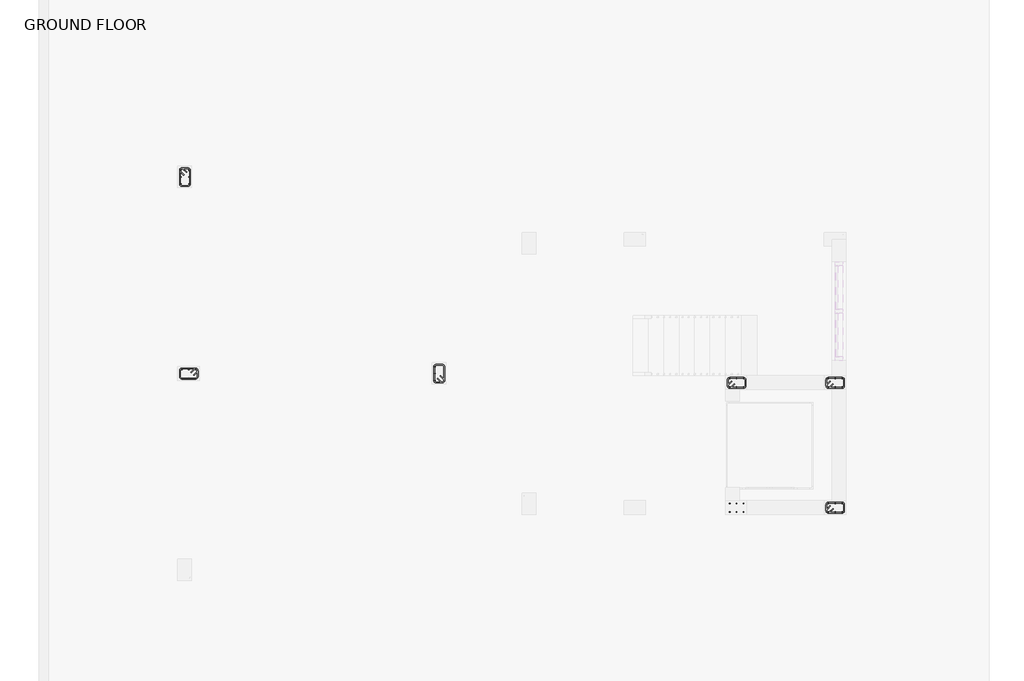
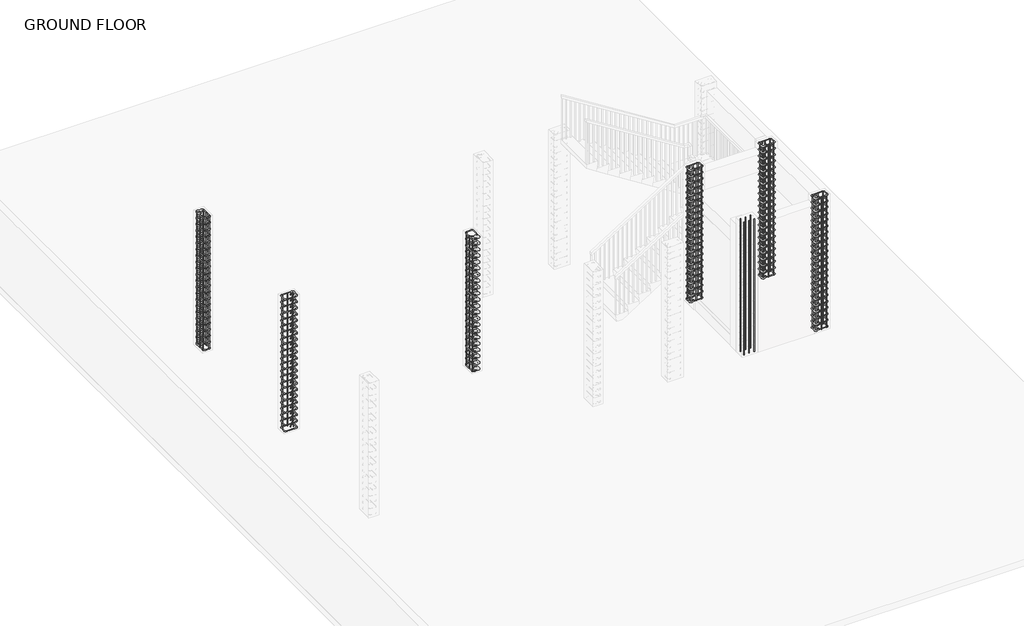
# One storey, part 5 of 7: 18 reinforcing bars.
"""IFC4 building model written with IfcOpenShell, lengths in millimetres."""

from ifc_helpers import new_model, si_unit, point, frame, origin, place, context, project, spatial, polyline, circle_curve, trimmed, segment, composite_curve, source, transform, mapped, element, save
from ifc_brep_helpers import swept_disk

model = new_model("IFC4")

# Units and contexts
model_context = context("Model", 3, world=origin())
ifc_project = project(units=[si_unit("LENGTHUNIT", "METRE", prefix="MILLI")], contexts=[model_context])

# Site, building, storey
site = spatial("IfcSite", under=ifc_project)
building = spatial("IfcBuilding", under=site)
storey = spatial("IfcBuildingStorey", under=building, Name="GROUND FLOOR", Elevation=0.0)

# Reinforcing bars
placement = place(None, origin())
reinforcing_bar_shape = source(origin(), model_context, "Body", "SolidModel", [
    swept_disk(composite_curve([segment(polyline([(4542.9487983, -124.2091695, 3168.65), (4489.0672616, -178.0907063, 3168.65)]), True, "CONTINUOUS"), segment(trimmed(circle_curve(frame((4466.6166213, -155.640066, 3168.65), z_axis=(0.0, 0.0, -1.0), x_axis=(22.450640300000487, -22.450640300000003, 0.0)), 31.75), [point((4489.0672616, -178.0907063, 3168.65))], [point((4434.8666213, -155.640066, 3168.65))], True, "CARTESIAN"), True, "CONTINUOUS"), segment(polyline([(4434.8666213, -155.640066, 3168.65), (4434.8666213, -54.040066, 3168.65)]), True, "CONTINUOUS"), segment(trimmed(circle_curve(frame((4466.6166213, -54.040066, 3168.65), z_axis=(0.0, 0.0, -1.0), x_axis=(-31.75, 0.0, 0.0)), 31.75), [point((4434.8666213, -54.040066, 3168.65))], [point((4466.6166213, -22.290066, 3168.65))], True, "CARTESIAN"), True, "CONTINUOUS"), segment(polyline([(4466.6166213, -22.290066, 3168.65), (4695.2166213, -22.290066, 3168.65)]), True, "CONTINUOUS"), segment(trimmed(circle_curve(frame((4695.2166213, -53.9465459, 3171.0851138), z_axis=(0.0, -0.07669649888473773, -0.9970544855015816), x_axis=(0.0, 31.656479899999997, -2.4351137999997263)), 31.75), [point((4695.2166213, -22.290066, 3168.65))], [point((4726.9666213, -53.9465459, 3171.0851138))], True, "CARTESIAN"), True, "CONTINUOUS"), segment(polyline([(4726.9666213, -53.9465459, 3171.0851138), (4726.9666213, -155.7335861, 3178.9148862)]), True, "CONTINUOUS"), segment(trimmed(circle_curve(frame((4695.2166213, -155.7335861, 3178.9148862), z_axis=(0.0, -0.07669649888473773, -0.9970544855015816), x_axis=(31.75, 0.0, 0.0)), 31.75), [point((4726.9666213, -155.7335861, 3178.9148862))], [point((4695.2166213, -187.390066, 3181.35))], True, "CARTESIAN"), True, "CONTINUOUS"), segment(polyline([(4695.2166213, -187.390066, 3181.35), (4466.6166213, -187.390066, 3181.35)]), True, "CONTINUOUS"), segment(trimmed(circle_curve(frame((4466.6166213, -155.640066, 3181.35), z_axis=(0.0, 0.0, -1.0), x_axis=(0.0, -31.75, 0.0)), 31.75), [point((4466.6166213, -187.390066, 3181.35))], [point((4444.165981, -133.1894257, 3181.35))], True, "CARTESIAN"), True, "CONTINUOUS"), segment(polyline([(4444.165981, -133.1894257, 3181.35), (4498.0475177, -79.3078889, 3181.35)]), True, "CONTINUOUS")], self_intersect=False), 6.35),
])
element("IfcReinforcingBar", 1, at=placement, inside=storey, context=model_context, shape_type="MappedRepresentation", body=[
    mapped(reinforcing_bar_shape, transform((0.0, 0.0, 0.0), x_axis=(1.0, 0.0, 0.0), y_axis=(0.0, 1.0, 0.0), z_axis=(0.0, 0.0, 1.0))),
    mapped(reinforcing_bar_shape, transform((0.0, 0.0, -149.3761905), x_axis=(1.0, 0.0, 0.0), y_axis=(0.0, 1.0, 0.0), z_axis=(0.0, 0.0, 1.0))),
    mapped(reinforcing_bar_shape, transform((0.0, 0.0, -298.752381), x_axis=(1.0, 0.0, 0.0), y_axis=(0.0, 1.0, 0.0), z_axis=(0.0, 0.0, 1.0))),
    mapped(reinforcing_bar_shape, transform((0.0, 0.0, -448.1285714), x_axis=(1.0, 0.0, 0.0), y_axis=(0.0, 1.0, 0.0), z_axis=(0.0, 0.0, 1.0))),
    mapped(reinforcing_bar_shape, transform((0.0, 0.0, -597.5047619), x_axis=(1.0, 0.0, 0.0), y_axis=(0.0, 1.0, 0.0), z_axis=(0.0, 0.0, 1.0))),
    mapped(reinforcing_bar_shape, transform((0.0, 0.0, -746.8809524), x_axis=(1.0, 0.0, 0.0), y_axis=(0.0, 1.0, 0.0), z_axis=(0.0, 0.0, 1.0))),
    mapped(reinforcing_bar_shape, transform((0.0, 0.0, -896.2571429), x_axis=(1.0, 0.0, 0.0), y_axis=(0.0, 1.0, 0.0), z_axis=(0.0, 0.0, 1.0))),
    mapped(reinforcing_bar_shape, transform((0.0, 0.0, -1045.6333333), x_axis=(1.0, 0.0, 0.0), y_axis=(0.0, 1.0, 0.0), z_axis=(0.0, 0.0, 1.0))),
    mapped(reinforcing_bar_shape, transform((0.0, 0.0, -1195.0095238), x_axis=(1.0, 0.0, 0.0), y_axis=(0.0, 1.0, 0.0), z_axis=(0.0, 0.0, 1.0))),
    mapped(reinforcing_bar_shape, transform((0.0, 0.0, -1344.3857143), x_axis=(1.0, 0.0, 0.0), y_axis=(0.0, 1.0, 0.0), z_axis=(0.0, 0.0, 1.0))),
    mapped(reinforcing_bar_shape, transform((0.0, 0.0, -1493.7619048), x_axis=(1.0, 0.0, 0.0), y_axis=(0.0, 1.0, 0.0), z_axis=(0.0, 0.0, 1.0))),
    mapped(reinforcing_bar_shape, transform((0.0, 0.0, -1643.1380952), x_axis=(1.0, 0.0, 0.0), y_axis=(0.0, 1.0, 0.0), z_axis=(0.0, 0.0, 1.0))),
    mapped(reinforcing_bar_shape, transform((0.0, 0.0, -1792.5142857), x_axis=(1.0, 0.0, 0.0), y_axis=(0.0, 1.0, 0.0), z_axis=(0.0, 0.0, 1.0))),
    mapped(reinforcing_bar_shape, transform((0.0, 0.0, -1941.8904762), x_axis=(1.0, 0.0, 0.0), y_axis=(0.0, 1.0, 0.0), z_axis=(0.0, 0.0, 1.0))),
    mapped(reinforcing_bar_shape, transform((0.0, 0.0, -2091.2666667), x_axis=(1.0, 0.0, 0.0), y_axis=(0.0, 1.0, 0.0), z_axis=(0.0, 0.0, 1.0))),
    mapped(reinforcing_bar_shape, transform((0.0, 0.0, -2240.6428571), x_axis=(1.0, 0.0, 0.0), y_axis=(0.0, 1.0, 0.0), z_axis=(0.0, 0.0, 1.0))),
    mapped(reinforcing_bar_shape, transform((0.0, 0.0, -2390.0190476), x_axis=(1.0, 0.0, 0.0), y_axis=(0.0, 1.0, 0.0), z_axis=(0.0, 0.0, 1.0))),
    mapped(reinforcing_bar_shape, transform((0.0, 0.0, -2539.3952381), x_axis=(1.0, 0.0, 0.0), y_axis=(0.0, 1.0, 0.0), z_axis=(0.0, 0.0, 1.0))),
    mapped(reinforcing_bar_shape, transform((0.0, 0.0, -2688.7714286), x_axis=(1.0, 0.0, 0.0), y_axis=(0.0, 1.0, 0.0), z_axis=(0.0, 0.0, 1.0))),
    mapped(reinforcing_bar_shape, transform((0.0, 0.0, -2838.147619), x_axis=(1.0, 0.0, 0.0), y_axis=(0.0, 1.0, 0.0), z_axis=(0.0, 0.0, 1.0))),
    mapped(reinforcing_bar_shape, transform((0.0, 0.0, -2987.5238095), x_axis=(1.0, 0.0, 0.0), y_axis=(0.0, 1.0, 0.0), z_axis=(0.0, 0.0, 1.0))),
    mapped(reinforcing_bar_shape, transform((0.0, 0.0, -3136.9), x_axis=(1.0, 0.0, 0.0), y_axis=(0.0, 1.0, 0.0), z_axis=(0.0, 0.0, 1.0))),
])
reinforcing_bar_2_shape = source(origin(), model_context, "Body", "SolidModel", [
    swept_disk(composite_curve([segment(polyline([(4466.6166213, -34.990066, 3175.0), (4466.6166213, -34.990066, 25.4)]), True, "CONTINUOUS")], self_intersect=False), 6.35),
])
element("IfcReinforcingBar", 2, at=placement, inside=storey, context=model_context, shape_type="MappedRepresentation", body=[
    mapped(reinforcing_bar_2_shape, transform((0.0, 0.0, 0.0), x_axis=(1.0, 0.0, 0.0), y_axis=(0.0, 1.0, 0.0), z_axis=(0.0, 0.0, 1.0))),
    mapped(reinforcing_bar_2_shape, transform((114.3, 0.0, 0.0), x_axis=(1.0, 0.0, 0.0), y_axis=(0.0, 1.0, 0.0), z_axis=(0.0, 0.0, 1.0))),
    mapped(reinforcing_bar_2_shape, transform((228.6, 0.0, 0.0), x_axis=(1.0, 0.0, 0.0), y_axis=(0.0, 1.0, 0.0), z_axis=(0.0, 0.0, 1.0))),
])
reinforcing_bar_3_shape = source(origin(), model_context, "Body", "SolidModel", [
    swept_disk(composite_curve([segment(polyline([(4466.6166213, -174.690066, 25.4), (4466.6166213, -174.690066, 3175.0)]), True, "CONTINUOUS")], self_intersect=False), 6.35),
])
element("IfcReinforcingBar", 3, at=placement, inside=storey, context=model_context, shape_type="MappedRepresentation", body=[
    mapped(reinforcing_bar_3_shape, transform((0.0, 0.0, 0.0), x_axis=(1.0, 0.0, 0.0), y_axis=(0.0, 1.0, 0.0), z_axis=(0.0, 0.0, 1.0))),
    mapped(reinforcing_bar_3_shape, transform((114.3, 0.0, 0.0), x_axis=(1.0, 0.0, 0.0), y_axis=(0.0, 1.0, 0.0), z_axis=(0.0, 0.0, 1.0))),
    mapped(reinforcing_bar_3_shape, transform((228.6, 0.0, 0.0), x_axis=(1.0, 0.0, 0.0), y_axis=(0.0, 1.0, 0.0), z_axis=(0.0, 0.0, 1.0))),
])
reinforcing_bar_4_shape = source(origin(), model_context, "Body", "SolidModel", [
    swept_disk(composite_curve([segment(polyline([(2917.3487983, -124.2091695, 3168.65), (2863.4672616, -178.0907063, 3168.65)]), True, "CONTINUOUS"), segment(trimmed(circle_curve(frame((2841.0166213, -155.640066, 3168.65), z_axis=(0.0, 0.0, -1.0), x_axis=(22.450640299999577, -22.450640300000003, 0.0)), 31.75), [point((2863.4672616, -178.0907063, 3168.65))], [point((2809.2666213, -155.640066, 3168.65))], True, "CARTESIAN"), True, "CONTINUOUS"), segment(polyline([(2809.2666213, -155.640066, 3168.65), (2809.2666213, -54.040066, 3168.65)]), True, "CONTINUOUS"), segment(trimmed(circle_curve(frame((2841.0166213, -54.040066, 3168.65), z_axis=(0.0, 0.0, -1.0), x_axis=(-31.75, 0.0, 0.0)), 31.75), [point((2809.2666213, -54.040066, 3168.65))], [point((2841.0166213, -22.290066, 3168.65))], True, "CARTESIAN"), True, "CONTINUOUS"), segment(polyline([(2841.0166213, -22.290066, 3168.65), (3069.6166213, -22.290066, 3168.65)]), True, "CONTINUOUS"), segment(trimmed(circle_curve(frame((3069.6166213, -53.9465459, 3171.0851138), z_axis=(0.0, -0.07669649888473773, -0.9970544855015816), x_axis=(0.0, 31.656479899999997, -2.4351137999997263)), 31.75), [point((3069.6166213, -22.290066, 3168.65))], [point((3101.3666213, -53.9465459, 3171.0851138))], True, "CARTESIAN"), True, "CONTINUOUS"), segment(polyline([(3101.3666213, -53.9465459, 3171.0851138), (3101.3666213, -155.7335861, 3178.9148862)]), True, "CONTINUOUS"), segment(trimmed(circle_curve(frame((3069.6166213, -155.7335861, 3178.9148862), z_axis=(0.0, -0.07669649888473773, -0.9970544855015816), x_axis=(31.75, 0.0, 0.0)), 31.75), [point((3101.3666213, -155.7335861, 3178.9148862))], [point((3069.6166213, -187.390066, 3181.35))], True, "CARTESIAN"), True, "CONTINUOUS"), segment(polyline([(3069.6166213, -187.390066, 3181.35), (2841.0166213, -187.390066, 3181.35)]), True, "CONTINUOUS"), segment(trimmed(circle_curve(frame((2841.0166213, -155.640066, 3181.35), z_axis=(0.0, 0.0, -1.0), x_axis=(0.0, -31.75, 0.0)), 31.75), [point((2841.0166213, -187.390066, 3181.35))], [point((2818.565981, -133.1894257, 3181.35))], True, "CARTESIAN"), True, "CONTINUOUS"), segment(polyline([(2818.565981, -133.1894257, 3181.35), (2872.4475177, -79.3078889, 3181.35)]), True, "CONTINUOUS")], self_intersect=False), 6.35),
])
element("IfcReinforcingBar", 4, at=placement, inside=storey, context=model_context, shape_type="MappedRepresentation", body=[
    mapped(reinforcing_bar_4_shape, transform((0.0, 0.0, 0.0), x_axis=(1.0, 0.0, 0.0), y_axis=(0.0, 1.0, 0.0), z_axis=(0.0, 0.0, 1.0))),
    mapped(reinforcing_bar_4_shape, transform((0.0, 0.0, -149.3761905), x_axis=(1.0, 0.0, 0.0), y_axis=(0.0, 1.0, 0.0), z_axis=(0.0, 0.0, 1.0))),
    mapped(reinforcing_bar_4_shape, transform((0.0, 0.0, -298.752381), x_axis=(1.0, 0.0, 0.0), y_axis=(0.0, 1.0, 0.0), z_axis=(0.0, 0.0, 1.0))),
    mapped(reinforcing_bar_4_shape, transform((0.0, 0.0, -448.1285714), x_axis=(1.0, 0.0, 0.0), y_axis=(0.0, 1.0, 0.0), z_axis=(0.0, 0.0, 1.0))),
    mapped(reinforcing_bar_4_shape, transform((0.0, 0.0, -597.5047619), x_axis=(1.0, 0.0, 0.0), y_axis=(0.0, 1.0, 0.0), z_axis=(0.0, 0.0, 1.0))),
    mapped(reinforcing_bar_4_shape, transform((0.0, 0.0, -746.8809524), x_axis=(1.0, 0.0, 0.0), y_axis=(0.0, 1.0, 0.0), z_axis=(0.0, 0.0, 1.0))),
    mapped(reinforcing_bar_4_shape, transform((0.0, 0.0, -896.2571429), x_axis=(1.0, 0.0, 0.0), y_axis=(0.0, 1.0, 0.0), z_axis=(0.0, 0.0, 1.0))),
    mapped(reinforcing_bar_4_shape, transform((0.0, 0.0, -1045.6333333), x_axis=(1.0, 0.0, 0.0), y_axis=(0.0, 1.0, 0.0), z_axis=(0.0, 0.0, 1.0))),
    mapped(reinforcing_bar_4_shape, transform((0.0, 0.0, -1195.0095238), x_axis=(1.0, 0.0, 0.0), y_axis=(0.0, 1.0, 0.0), z_axis=(0.0, 0.0, 1.0))),
    mapped(reinforcing_bar_4_shape, transform((0.0, 0.0, -1344.3857143), x_axis=(1.0, 0.0, 0.0), y_axis=(0.0, 1.0, 0.0), z_axis=(0.0, 0.0, 1.0))),
    mapped(reinforcing_bar_4_shape, transform((0.0, 0.0, -1493.7619048), x_axis=(1.0, 0.0, 0.0), y_axis=(0.0, 1.0, 0.0), z_axis=(0.0, 0.0, 1.0))),
    mapped(reinforcing_bar_4_shape, transform((0.0, 0.0, -1643.1380952), x_axis=(1.0, 0.0, 0.0), y_axis=(0.0, 1.0, 0.0), z_axis=(0.0, 0.0, 1.0))),
    mapped(reinforcing_bar_4_shape, transform((0.0, 0.0, -1792.5142857), x_axis=(1.0, 0.0, 0.0), y_axis=(0.0, 1.0, 0.0), z_axis=(0.0, 0.0, 1.0))),
    mapped(reinforcing_bar_4_shape, transform((0.0, 0.0, -1941.8904762), x_axis=(1.0, 0.0, 0.0), y_axis=(0.0, 1.0, 0.0), z_axis=(0.0, 0.0, 1.0))),
    mapped(reinforcing_bar_4_shape, transform((0.0, 0.0, -2091.2666667), x_axis=(1.0, 0.0, 0.0), y_axis=(0.0, 1.0, 0.0), z_axis=(0.0, 0.0, 1.0))),
    mapped(reinforcing_bar_4_shape, transform((0.0, 0.0, -2240.6428571), x_axis=(1.0, 0.0, 0.0), y_axis=(0.0, 1.0, 0.0), z_axis=(0.0, 0.0, 1.0))),
    mapped(reinforcing_bar_4_shape, transform((0.0, 0.0, -2390.0190476), x_axis=(1.0, 0.0, 0.0), y_axis=(0.0, 1.0, 0.0), z_axis=(0.0, 0.0, 1.0))),
    mapped(reinforcing_bar_4_shape, transform((0.0, 0.0, -2539.3952381), x_axis=(1.0, 0.0, 0.0), y_axis=(0.0, 1.0, 0.0), z_axis=(0.0, 0.0, 1.0))),
    mapped(reinforcing_bar_4_shape, transform((0.0, 0.0, -2688.7714286), x_axis=(1.0, 0.0, 0.0), y_axis=(0.0, 1.0, 0.0), z_axis=(0.0, 0.0, 1.0))),
    mapped(reinforcing_bar_4_shape, transform((0.0, 0.0, -2838.147619), x_axis=(1.0, 0.0, 0.0), y_axis=(0.0, 1.0, 0.0), z_axis=(0.0, 0.0, 1.0))),
    mapped(reinforcing_bar_4_shape, transform((0.0, 0.0, -2987.5238095), x_axis=(1.0, 0.0, 0.0), y_axis=(0.0, 1.0, 0.0), z_axis=(0.0, 0.0, 1.0))),
    mapped(reinforcing_bar_4_shape, transform((0.0, 0.0, -3136.9), x_axis=(1.0, 0.0, 0.0), y_axis=(0.0, 1.0, 0.0), z_axis=(0.0, 0.0, 1.0))),
])
reinforcing_bar_5_shape = source(origin(), model_context, "Body", "SolidModel", [
    swept_disk(composite_curve([segment(polyline([(2841.0166213, -34.990066, 3175.0), (2841.0166213, -34.990066, 25.4)]), True, "CONTINUOUS")], self_intersect=False), 6.35),
])
element("IfcReinforcingBar", 5, at=placement, inside=storey, context=model_context, shape_type="MappedRepresentation", body=[
    mapped(reinforcing_bar_5_shape, transform((0.0, 0.0, 0.0), x_axis=(1.0, 0.0, 0.0), y_axis=(0.0, 1.0, 0.0), z_axis=(0.0, 0.0, 1.0))),
    mapped(reinforcing_bar_5_shape, transform((114.3, 0.0, 0.0), x_axis=(1.0, 0.0, 0.0), y_axis=(0.0, 1.0, 0.0), z_axis=(0.0, 0.0, 1.0))),
    mapped(reinforcing_bar_5_shape, transform((228.6, 0.0, 0.0), x_axis=(1.0, 0.0, 0.0), y_axis=(0.0, 1.0, 0.0), z_axis=(0.0, 0.0, 1.0))),
])
reinforcing_bar_6_shape = source(origin(), model_context, "Body", "SolidModel", [
    swept_disk(composite_curve([segment(polyline([(2841.0166213, -174.690066, 25.4), (2841.0166213, -174.690066, 3175.0)]), True, "CONTINUOUS")], self_intersect=False), 6.35),
])
element("IfcReinforcingBar", 6, at=placement, inside=storey, context=model_context, shape_type="MappedRepresentation", body=[
    mapped(reinforcing_bar_6_shape, transform((0.0, 0.0, 0.0), x_axis=(1.0, 0.0, 0.0), y_axis=(0.0, 1.0, 0.0), z_axis=(0.0, 0.0, 1.0))),
    mapped(reinforcing_bar_6_shape, transform((114.3, 0.0, 0.0), x_axis=(1.0, 0.0, 0.0), y_axis=(0.0, 1.0, 0.0), z_axis=(0.0, 0.0, 1.0))),
    mapped(reinforcing_bar_6_shape, transform((228.6, 0.0, 0.0), x_axis=(1.0, 0.0, 0.0), y_axis=(0.0, 1.0, 0.0), z_axis=(0.0, 0.0, 1.0))),
])
reinforcing_bar_7_shape = source(origin(), model_context, "Body", "SolidModel", [
    swept_disk(composite_curve([segment(polyline([(4542.9487983, -2181.6091695, 3168.65), (4489.0672616, -2235.4907063, 3168.65)]), True, "CONTINUOUS"), segment(trimmed(circle_curve(frame((4466.6166213, -2213.040066, 3168.65), z_axis=(0.0, 0.0, -1.0), x_axis=(22.450640300000487, -22.450640300000032, 0.0)), 31.75), [point((4489.0672616, -2235.4907063, 3168.65))], [point((4434.8666213, -2213.040066, 3168.65))], True, "CARTESIAN"), True, "CONTINUOUS"), segment(polyline([(4434.8666213, -2213.040066, 3168.65), (4434.8666213, -2111.440066, 3168.65)]), True, "CONTINUOUS"), segment(trimmed(circle_curve(frame((4466.6166213, -2111.440066, 3168.65), z_axis=(0.0, 0.0, -1.0), x_axis=(-31.75, 0.0, 0.0)), 31.75), [point((4434.8666213, -2111.440066, 3168.65))], [point((4466.6166213, -2079.690066, 3168.65))], True, "CARTESIAN"), True, "CONTINUOUS"), segment(polyline([(4466.6166213, -2079.690066, 3168.65), (4695.2166213, -2079.690066, 3168.65)]), True, "CONTINUOUS"), segment(trimmed(circle_curve(frame((4695.2166213, -2111.3465459, 3171.0851138), z_axis=(0.0, -0.07669649888473773, -0.9970544855015816), x_axis=(0.0, 31.656479899999795, -2.4351137999997263)), 31.75), [point((4695.2166213, -2079.690066, 3168.65))], [point((4726.9666213, -2111.3465459, 3171.0851138))], True, "CARTESIAN"), True, "CONTINUOUS"), segment(polyline([(4726.9666213, -2111.3465459, 3171.0851138), (4726.9666213, -2213.1335861, 3178.9148862)]), True, "CONTINUOUS"), segment(trimmed(circle_curve(frame((4695.2166213, -2213.1335861, 3178.9148862), z_axis=(0.0, -0.07669649888473773, -0.9970544855015816), x_axis=(31.75, 0.0, 0.0)), 31.75), [point((4726.9666213, -2213.1335861, 3178.9148862))], [point((4695.2166213, -2244.790066, 3181.35))], True, "CARTESIAN"), True, "CONTINUOUS"), segment(polyline([(4695.2166213, -2244.790066, 3181.35), (4466.6166213, -2244.790066, 3181.35)]), True, "CONTINUOUS"), segment(trimmed(circle_curve(frame((4466.6166213, -2213.040066, 3181.35), z_axis=(0.0, 0.0, -1.0), x_axis=(0.0, -31.75, 0.0)), 31.75), [point((4466.6166213, -2244.790066, 3181.35))], [point((4444.165981, -2190.5894257, 3181.35))], True, "CARTESIAN"), True, "CONTINUOUS"), segment(polyline([(4444.165981, -2190.5894257, 3181.35), (4498.0475177, -2136.7078889, 3181.35)]), True, "CONTINUOUS")], self_intersect=False), 6.35),
])
element("IfcReinforcingBar", 7, at=placement, inside=storey, context=model_context, shape_type="MappedRepresentation", body=[
    mapped(reinforcing_bar_7_shape, transform((0.0, 0.0, 0.0), x_axis=(1.0, 0.0, 0.0), y_axis=(0.0, 1.0, 0.0), z_axis=(0.0, 0.0, 1.0))),
    mapped(reinforcing_bar_7_shape, transform((0.0, 0.0, -149.3761905), x_axis=(1.0, 0.0, 0.0), y_axis=(0.0, 1.0, 0.0), z_axis=(0.0, 0.0, 1.0))),
    mapped(reinforcing_bar_7_shape, transform((0.0, 0.0, -298.752381), x_axis=(1.0, 0.0, 0.0), y_axis=(0.0, 1.0, 0.0), z_axis=(0.0, 0.0, 1.0))),
    mapped(reinforcing_bar_7_shape, transform((0.0, 0.0, -448.1285714), x_axis=(1.0, 0.0, 0.0), y_axis=(0.0, 1.0, 0.0), z_axis=(0.0, 0.0, 1.0))),
    mapped(reinforcing_bar_7_shape, transform((0.0, 0.0, -597.5047619), x_axis=(1.0, 0.0, 0.0), y_axis=(0.0, 1.0, 0.0), z_axis=(0.0, 0.0, 1.0))),
    mapped(reinforcing_bar_7_shape, transform((0.0, 0.0, -746.8809524), x_axis=(1.0, 0.0, 0.0), y_axis=(0.0, 1.0, 0.0), z_axis=(0.0, 0.0, 1.0))),
    mapped(reinforcing_bar_7_shape, transform((0.0, 0.0, -896.2571429), x_axis=(1.0, 0.0, 0.0), y_axis=(0.0, 1.0, 0.0), z_axis=(0.0, 0.0, 1.0))),
    mapped(reinforcing_bar_7_shape, transform((0.0, 0.0, -1045.6333333), x_axis=(1.0, 0.0, 0.0), y_axis=(0.0, 1.0, 0.0), z_axis=(0.0, 0.0, 1.0))),
    mapped(reinforcing_bar_7_shape, transform((0.0, 0.0, -1195.0095238), x_axis=(1.0, 0.0, 0.0), y_axis=(0.0, 1.0, 0.0), z_axis=(0.0, 0.0, 1.0))),
    mapped(reinforcing_bar_7_shape, transform((0.0, 0.0, -1344.3857143), x_axis=(1.0, 0.0, 0.0), y_axis=(0.0, 1.0, 0.0), z_axis=(0.0, 0.0, 1.0))),
    mapped(reinforcing_bar_7_shape, transform((0.0, 0.0, -1493.7619048), x_axis=(1.0, 0.0, 0.0), y_axis=(0.0, 1.0, 0.0), z_axis=(0.0, 0.0, 1.0))),
    mapped(reinforcing_bar_7_shape, transform((0.0, 0.0, -1643.1380952), x_axis=(1.0, 0.0, 0.0), y_axis=(0.0, 1.0, 0.0), z_axis=(0.0, 0.0, 1.0))),
    mapped(reinforcing_bar_7_shape, transform((0.0, 0.0, -1792.5142857), x_axis=(1.0, 0.0, 0.0), y_axis=(0.0, 1.0, 0.0), z_axis=(0.0, 0.0, 1.0))),
    mapped(reinforcing_bar_7_shape, transform((0.0, 0.0, -1941.8904762), x_axis=(1.0, 0.0, 0.0), y_axis=(0.0, 1.0, 0.0), z_axis=(0.0, 0.0, 1.0))),
    mapped(reinforcing_bar_7_shape, transform((0.0, 0.0, -2091.2666667), x_axis=(1.0, 0.0, 0.0), y_axis=(0.0, 1.0, 0.0), z_axis=(0.0, 0.0, 1.0))),
    mapped(reinforcing_bar_7_shape, transform((0.0, 0.0, -2240.6428571), x_axis=(1.0, 0.0, 0.0), y_axis=(0.0, 1.0, 0.0), z_axis=(0.0, 0.0, 1.0))),
    mapped(reinforcing_bar_7_shape, transform((0.0, 0.0, -2390.0190476), x_axis=(1.0, 0.0, 0.0), y_axis=(0.0, 1.0, 0.0), z_axis=(0.0, 0.0, 1.0))),
    mapped(reinforcing_bar_7_shape, transform((0.0, 0.0, -2539.3952381), x_axis=(1.0, 0.0, 0.0), y_axis=(0.0, 1.0, 0.0), z_axis=(0.0, 0.0, 1.0))),
    mapped(reinforcing_bar_7_shape, transform((0.0, 0.0, -2688.7714286), x_axis=(1.0, 0.0, 0.0), y_axis=(0.0, 1.0, 0.0), z_axis=(0.0, 0.0, 1.0))),
    mapped(reinforcing_bar_7_shape, transform((0.0, 0.0, -2838.147619), x_axis=(1.0, 0.0, 0.0), y_axis=(0.0, 1.0, 0.0), z_axis=(0.0, 0.0, 1.0))),
    mapped(reinforcing_bar_7_shape, transform((0.0, 0.0, -2987.5238095), x_axis=(1.0, 0.0, 0.0), y_axis=(0.0, 1.0, 0.0), z_axis=(0.0, 0.0, 1.0))),
    mapped(reinforcing_bar_7_shape, transform((0.0, 0.0, -3136.9), x_axis=(1.0, 0.0, 0.0), y_axis=(0.0, 1.0, 0.0), z_axis=(0.0, 0.0, 1.0))),
])
reinforcing_bar_8_shape = source(origin(), model_context, "Body", "SolidModel", [
    swept_disk(composite_curve([segment(polyline([(4466.6166213, -2092.390066, 3175.0), (4466.6166213, -2092.390066, 25.4)]), True, "CONTINUOUS")], self_intersect=False), 6.35),
])
element("IfcReinforcingBar", 8, at=placement, inside=storey, context=model_context, shape_type="MappedRepresentation", body=[
    mapped(reinforcing_bar_8_shape, transform((0.0, 0.0, 0.0), x_axis=(1.0, 0.0, 0.0), y_axis=(0.0, 1.0, 0.0), z_axis=(0.0, 0.0, 1.0))),
    mapped(reinforcing_bar_8_shape, transform((114.3, 0.0, 0.0), x_axis=(1.0, 0.0, 0.0), y_axis=(0.0, 1.0, 0.0), z_axis=(0.0, 0.0, 1.0))),
    mapped(reinforcing_bar_8_shape, transform((228.6, 0.0, 0.0), x_axis=(1.0, 0.0, 0.0), y_axis=(0.0, 1.0, 0.0), z_axis=(0.0, 0.0, 1.0))),
])
reinforcing_bar_9_shape = source(origin(), model_context, "Body", "SolidModel", [
    swept_disk(composite_curve([segment(polyline([(4466.6166213, -2232.090066, 25.4), (4466.6166213, -2232.090066, 3175.0)]), True, "CONTINUOUS")], self_intersect=False), 6.35),
])
element("IfcReinforcingBar", 9, at=placement, inside=storey, context=model_context, shape_type="MappedRepresentation", body=[
    mapped(reinforcing_bar_9_shape, transform((0.0, 0.0, 0.0), x_axis=(1.0, 0.0, 0.0), y_axis=(0.0, 1.0, 0.0), z_axis=(0.0, 0.0, 1.0))),
    mapped(reinforcing_bar_9_shape, transform((114.3, 0.0, 0.0), x_axis=(1.0, 0.0, 0.0), y_axis=(0.0, 1.0, 0.0), z_axis=(0.0, 0.0, 1.0))),
    mapped(reinforcing_bar_9_shape, transform((228.6, 0.0, 0.0), x_axis=(1.0, 0.0, 0.0), y_axis=(0.0, 1.0, 0.0), z_axis=(0.0, 0.0, 1.0))),
])
reinforcing_bar_10_shape = source(origin(), model_context, "Body", "SolidModel", [
    swept_disk(composite_curve([segment(polyline([(2841.0166213, -2092.390066, 3175.0), (2841.0166213, -2092.390066, 25.4)]), True, "CONTINUOUS")], self_intersect=False), 6.35),
])
element("IfcReinforcingBar", 10, at=placement, inside=storey, context=model_context, shape_type="MappedRepresentation", body=[
    mapped(reinforcing_bar_10_shape, transform((0.0, 0.0, 0.0), x_axis=(1.0, 0.0, 0.0), y_axis=(0.0, 1.0, 0.0), z_axis=(0.0, 0.0, 1.0))),
    mapped(reinforcing_bar_10_shape, transform((114.3, 0.0, 0.0), x_axis=(1.0, 0.0, 0.0), y_axis=(0.0, 1.0, 0.0), z_axis=(0.0, 0.0, 1.0))),
    mapped(reinforcing_bar_10_shape, transform((228.6, 0.0, 0.0), x_axis=(1.0, 0.0, 0.0), y_axis=(0.0, 1.0, 0.0), z_axis=(0.0, 0.0, 1.0))),
])
reinforcing_bar_11_shape = source(origin(), model_context, "Body", "SolidModel", [
    swept_disk(composite_curve([segment(polyline([(2841.0166213, -2232.090066, 25.4), (2841.0166213, -2232.090066, 3175.0)]), True, "CONTINUOUS")], self_intersect=False), 6.35),
])
element("IfcReinforcingBar", 11, at=placement, inside=storey, context=model_context, shape_type="MappedRepresentation", body=[
    mapped(reinforcing_bar_11_shape, transform((0.0, 0.0, 0.0), x_axis=(1.0, 0.0, 0.0), y_axis=(0.0, 1.0, 0.0), z_axis=(0.0, 0.0, 1.0))),
    mapped(reinforcing_bar_11_shape, transform((114.3, 0.0, 0.0), x_axis=(1.0, 0.0, 0.0), y_axis=(0.0, 1.0, 0.0), z_axis=(0.0, 0.0, 1.0))),
    mapped(reinforcing_bar_11_shape, transform((228.6, 0.0, 0.0), x_axis=(1.0, 0.0, 0.0), y_axis=(0.0, 1.0, 0.0), z_axis=(0.0, 0.0, 1.0))),
])
reinforcing_bar_12_shape = source(origin(), model_context, "Body", "SolidModel", [
    swept_disk(composite_curve([segment(polyline([(-1927.5142752, 9.5921111, 3168.65), (-1873.6327384, -44.2894257, 3168.65)]), True, "CONTINUOUS"), segment(trimmed(circle_curve(frame((-1896.0833787, -66.740066, 3168.65), z_axis=(0.0, 0.0, -1.0), x_axis=(22.450640299999804, 22.450640299999996, 0.0)), 31.75), [point((-1873.6327384, -44.2894257, 3168.65))], [point((-1896.0833787, -98.490066, 3168.65))], True, "CARTESIAN"), True, "CONTINUOUS"), segment(polyline([(-1896.0833787, -98.490066, 3168.65), (-1997.6833787, -98.490066, 3168.65)]), True, "CONTINUOUS"), segment(trimmed(circle_curve(frame((-1997.6833787, -66.740066, 3168.65), z_axis=(0.0, 0.0, -1.0), x_axis=(0.0, -31.75, 0.0)), 31.75), [point((-1997.6833787, -98.490066, 3168.65))], [point((-2029.4333787, -66.740066, 3168.65))], True, "CARTESIAN"), True, "CONTINUOUS"), segment(polyline([(-2029.4333787, -66.740066, 3168.65), (-2029.4333787, 161.859934, 3168.65)]), True, "CONTINUOUS"), segment(trimmed(circle_curve(frame((-1997.7768988, 161.859934, 3171.0851138), z_axis=(0.07669649888473773, 0.0, -0.9970544855015816), x_axis=(-31.656479900000022, 0.0, -2.4351137999997263)), 31.75), [point((-2029.4333787, 161.859934, 3168.65))], [point((-1997.7768988, 193.609934, 3171.0851138))], True, "CARTESIAN"), True, "CONTINUOUS"), segment(polyline([(-1997.7768988, 193.609934, 3171.0851138), (-1895.9898586, 193.609934, 3178.9148862)]), True, "CONTINUOUS"), segment(trimmed(circle_curve(frame((-1895.9898586, 161.859934, 3178.9148862), z_axis=(0.07669649888473773, 0.0, -0.9970544855015816), x_axis=(0.0, 31.75, 0.0)), 31.75), [point((-1895.9898586, 193.609934, 3178.9148862))], [point((-1864.3333787, 161.859934, 3181.35))], True, "CARTESIAN"), True, "CONTINUOUS"), segment(polyline([(-1864.3333787, 161.859934, 3181.35), (-1864.3333787, -66.740066, 3181.35)]), True, "CONTINUOUS"), segment(trimmed(circle_curve(frame((-1896.0833787, -66.740066, 3181.35), z_axis=(0.0, 0.0, -1.0), x_axis=(31.75, 0.0, 0.0)), 31.75), [point((-1864.3333787, -66.740066, 3181.35))], [point((-1918.534019, -89.1907063, 3181.35))], True, "CARTESIAN"), True, "CONTINUOUS"), segment(polyline([(-1918.534019, -89.1907063, 3181.35), (-1972.4155558, -35.3091695, 3181.35)]), True, "CONTINUOUS")], self_intersect=False), 6.35),
])
element("IfcReinforcingBar", 12, at=placement, inside=storey, context=model_context, shape_type="MappedRepresentation", body=[
    mapped(reinforcing_bar_12_shape, transform((0.0, 0.0, 0.0), x_axis=(1.0, 0.0, 0.0), y_axis=(0.0, 1.0, 0.0), z_axis=(0.0, 0.0, 1.0))),
    mapped(reinforcing_bar_12_shape, transform((0.0, 0.0, -149.3761905), x_axis=(1.0, 0.0, 0.0), y_axis=(0.0, 1.0, 0.0), z_axis=(0.0, 0.0, 1.0))),
    mapped(reinforcing_bar_12_shape, transform((0.0, 0.0, -298.752381), x_axis=(1.0, 0.0, 0.0), y_axis=(0.0, 1.0, 0.0), z_axis=(0.0, 0.0, 1.0))),
    mapped(reinforcing_bar_12_shape, transform((0.0, 0.0, -448.1285714), x_axis=(1.0, 0.0, 0.0), y_axis=(0.0, 1.0, 0.0), z_axis=(0.0, 0.0, 1.0))),
    mapped(reinforcing_bar_12_shape, transform((0.0, 0.0, -597.5047619), x_axis=(1.0, 0.0, 0.0), y_axis=(0.0, 1.0, 0.0), z_axis=(0.0, 0.0, 1.0))),
    mapped(reinforcing_bar_12_shape, transform((0.0, 0.0, -746.8809524), x_axis=(1.0, 0.0, 0.0), y_axis=(0.0, 1.0, 0.0), z_axis=(0.0, 0.0, 1.0))),
    mapped(reinforcing_bar_12_shape, transform((0.0, 0.0, -896.2571429), x_axis=(1.0, 0.0, 0.0), y_axis=(0.0, 1.0, 0.0), z_axis=(0.0, 0.0, 1.0))),
    mapped(reinforcing_bar_12_shape, transform((0.0, 0.0, -1045.6333333), x_axis=(1.0, 0.0, 0.0), y_axis=(0.0, 1.0, 0.0), z_axis=(0.0, 0.0, 1.0))),
    mapped(reinforcing_bar_12_shape, transform((0.0, 0.0, -1195.0095238), x_axis=(1.0, 0.0, 0.0), y_axis=(0.0, 1.0, 0.0), z_axis=(0.0, 0.0, 1.0))),
    mapped(reinforcing_bar_12_shape, transform((0.0, 0.0, -1344.3857143), x_axis=(1.0, 0.0, 0.0), y_axis=(0.0, 1.0, 0.0), z_axis=(0.0, 0.0, 1.0))),
    mapped(reinforcing_bar_12_shape, transform((0.0, 0.0, -1493.7619048), x_axis=(1.0, 0.0, 0.0), y_axis=(0.0, 1.0, 0.0), z_axis=(0.0, 0.0, 1.0))),
    mapped(reinforcing_bar_12_shape, transform((0.0, 0.0, -1643.1380952), x_axis=(1.0, 0.0, 0.0), y_axis=(0.0, 1.0, 0.0), z_axis=(0.0, 0.0, 1.0))),
    mapped(reinforcing_bar_12_shape, transform((0.0, 0.0, -1792.5142857), x_axis=(1.0, 0.0, 0.0), y_axis=(0.0, 1.0, 0.0), z_axis=(0.0, 0.0, 1.0))),
    mapped(reinforcing_bar_12_shape, transform((0.0, 0.0, -1941.8904762), x_axis=(1.0, 0.0, 0.0), y_axis=(0.0, 1.0, 0.0), z_axis=(0.0, 0.0, 1.0))),
    mapped(reinforcing_bar_12_shape, transform((0.0, 0.0, -2091.2666667), x_axis=(1.0, 0.0, 0.0), y_axis=(0.0, 1.0, 0.0), z_axis=(0.0, 0.0, 1.0))),
    mapped(reinforcing_bar_12_shape, transform((0.0, 0.0, -2240.6428571), x_axis=(1.0, 0.0, 0.0), y_axis=(0.0, 1.0, 0.0), z_axis=(0.0, 0.0, 1.0))),
    mapped(reinforcing_bar_12_shape, transform((0.0, 0.0, -2390.0190476), x_axis=(1.0, 0.0, 0.0), y_axis=(0.0, 1.0, 0.0), z_axis=(0.0, 0.0, 1.0))),
    mapped(reinforcing_bar_12_shape, transform((0.0, 0.0, -2539.3952381), x_axis=(1.0, 0.0, 0.0), y_axis=(0.0, 1.0, 0.0), z_axis=(0.0, 0.0, 1.0))),
    mapped(reinforcing_bar_12_shape, transform((0.0, 0.0, -2688.7714286), x_axis=(1.0, 0.0, 0.0), y_axis=(0.0, 1.0, 0.0), z_axis=(0.0, 0.0, 1.0))),
    mapped(reinforcing_bar_12_shape, transform((0.0, 0.0, -2838.147619), x_axis=(1.0, 0.0, 0.0), y_axis=(0.0, 1.0, 0.0), z_axis=(0.0, 0.0, 1.0))),
    mapped(reinforcing_bar_12_shape, transform((0.0, 0.0, -2987.5238095), x_axis=(1.0, 0.0, 0.0), y_axis=(0.0, 1.0, 0.0), z_axis=(0.0, 0.0, 1.0))),
    mapped(reinforcing_bar_12_shape, transform((0.0, 0.0, -3136.9), x_axis=(1.0, 0.0, 0.0), y_axis=(0.0, 1.0, 0.0), z_axis=(0.0, 0.0, 1.0))),
])
reinforcing_bar_13_shape = source(origin(), model_context, "Body", "SolidModel", [
    swept_disk(composite_curve([segment(polyline([(-2016.7333787, -66.740066, 3175.0), (-2016.7333787, -66.740066, 25.4)]), True, "CONTINUOUS")], self_intersect=False), 6.35),
])
element("IfcReinforcingBar", 13, at=placement, inside=storey, context=model_context, shape_type="MappedRepresentation", body=[
    mapped(reinforcing_bar_13_shape, transform((0.0, 0.0, 0.0), x_axis=(1.0, 0.0, 0.0), y_axis=(0.0, 1.0, 0.0), z_axis=(0.0, 0.0, 1.0))),
    mapped(reinforcing_bar_13_shape, transform((0.0, 114.3, 0.0), x_axis=(1.0, 0.0, 0.0), y_axis=(0.0, 1.0, 0.0), z_axis=(0.0, 0.0, 1.0))),
    mapped(reinforcing_bar_13_shape, transform((0.0, 228.6, 0.0), x_axis=(1.0, 0.0, 0.0), y_axis=(0.0, 1.0, 0.0), z_axis=(0.0, 0.0, 1.0))),
])
reinforcing_bar_14_shape = source(origin(), model_context, "Body", "SolidModel", [
    swept_disk(composite_curve([segment(polyline([(-6157.2524823, 3324.027757, 3168.65), (-6211.134019, 3377.9092937, 3168.65)]), True, "CONTINUOUS"), segment(trimmed(circle_curve(frame((-6188.6833787, 3400.359934, 3168.65), z_axis=(0.0, 0.0, -1.0), x_axis=(-22.450640300000487, -22.450640300000032, 0.0)), 31.75), [point((-6211.134019, 3377.9092937, 3168.65))], [point((-6188.6833787, 3432.109934, 3168.65))], True, "CARTESIAN"), True, "CONTINUOUS"), segment(polyline([(-6188.6833787, 3432.109934, 3168.65), (-6087.0833787, 3432.109934, 3168.65)]), True, "CONTINUOUS"), segment(trimmed(circle_curve(frame((-6087.0833787, 3400.359934, 3168.65), z_axis=(0.0, 0.0, -1.0), x_axis=(0.0, 31.75, 0.0)), 31.75), [point((-6087.0833787, 3432.109934, 3168.65))], [point((-6055.3333787, 3400.359934, 3168.65))], True, "CARTESIAN"), True, "CONTINUOUS"), segment(polyline([(-6055.3333787, 3400.359934, 3168.65), (-6055.3333787, 3171.759934, 3168.65)]), True, "CONTINUOUS"), segment(trimmed(circle_curve(frame((-6086.9898586, 3171.759934, 3171.0851138), z_axis=(-0.07669649888473773, 0.0, -0.9970544855015816), x_axis=(31.656479899999795, 0.0, -2.4351137999997263)), 31.75), [point((-6055.3333787, 3171.759934, 3168.65))], [point((-6086.9898586, 3140.009934, 3171.0851138))], True, "CARTESIAN"), True, "CONTINUOUS"), segment(polyline([(-6086.9898586, 3140.009934, 3171.0851138), (-6188.7768988, 3140.009934, 3178.9148862)]), True, "CONTINUOUS"), segment(trimmed(circle_curve(frame((-6188.7768988, 3171.759934, 3178.9148862), z_axis=(-0.07669649888473773, 0.0, -0.9970544855015816), x_axis=(0.0, -31.75, 0.0)), 31.75), [point((-6188.7768988, 3140.009934, 3178.9148862))], [point((-6220.4333787, 3171.759934, 3181.35))], True, "CARTESIAN"), True, "CONTINUOUS"), segment(polyline([(-6220.4333787, 3171.759934, 3181.35), (-6220.4333787, 3400.359934, 3181.35)]), True, "CONTINUOUS"), segment(trimmed(circle_curve(frame((-6188.6833787, 3400.359934, 3181.35), z_axis=(0.0, 0.0, -1.0), x_axis=(-31.75, 0.0, 0.0)), 31.75), [point((-6220.4333787, 3400.359934, 3181.35))], [point((-6166.2327384, 3422.8105743, 3181.35))], True, "CARTESIAN"), True, "CONTINUOUS"), segment(polyline([(-6166.2327384, 3422.8105743, 3181.35), (-6112.3512017, 3368.9290376, 3181.35)]), True, "CONTINUOUS")], self_intersect=False), 6.35),
])
element("IfcReinforcingBar", 14, at=placement, inside=storey, context=model_context, shape_type="MappedRepresentation", body=[
    mapped(reinforcing_bar_14_shape, transform((0.0, 0.0, 0.0), x_axis=(1.0, 0.0, 0.0), y_axis=(0.0, 1.0, 0.0), z_axis=(0.0, 0.0, 1.0))),
    mapped(reinforcing_bar_14_shape, transform((0.0, 0.0, -149.3761905), x_axis=(1.0, 0.0, 0.0), y_axis=(0.0, 1.0, 0.0), z_axis=(0.0, 0.0, 1.0))),
    mapped(reinforcing_bar_14_shape, transform((0.0, 0.0, -298.752381), x_axis=(1.0, 0.0, 0.0), y_axis=(0.0, 1.0, 0.0), z_axis=(0.0, 0.0, 1.0))),
    mapped(reinforcing_bar_14_shape, transform((0.0, 0.0, -448.1285714), x_axis=(1.0, 0.0, 0.0), y_axis=(0.0, 1.0, 0.0), z_axis=(0.0, 0.0, 1.0))),
    mapped(reinforcing_bar_14_shape, transform((0.0, 0.0, -597.5047619), x_axis=(1.0, 0.0, 0.0), y_axis=(0.0, 1.0, 0.0), z_axis=(0.0, 0.0, 1.0))),
    mapped(reinforcing_bar_14_shape, transform((0.0, 0.0, -746.8809524), x_axis=(1.0, 0.0, 0.0), y_axis=(0.0, 1.0, 0.0), z_axis=(0.0, 0.0, 1.0))),
    mapped(reinforcing_bar_14_shape, transform((0.0, 0.0, -896.2571429), x_axis=(1.0, 0.0, 0.0), y_axis=(0.0, 1.0, 0.0), z_axis=(0.0, 0.0, 1.0))),
    mapped(reinforcing_bar_14_shape, transform((0.0, 0.0, -1045.6333333), x_axis=(1.0, 0.0, 0.0), y_axis=(0.0, 1.0, 0.0), z_axis=(0.0, 0.0, 1.0))),
    mapped(reinforcing_bar_14_shape, transform((0.0, 0.0, -1195.0095238), x_axis=(1.0, 0.0, 0.0), y_axis=(0.0, 1.0, 0.0), z_axis=(0.0, 0.0, 1.0))),
    mapped(reinforcing_bar_14_shape, transform((0.0, 0.0, -1344.3857143), x_axis=(1.0, 0.0, 0.0), y_axis=(0.0, 1.0, 0.0), z_axis=(0.0, 0.0, 1.0))),
    mapped(reinforcing_bar_14_shape, transform((0.0, 0.0, -1493.7619048), x_axis=(1.0, 0.0, 0.0), y_axis=(0.0, 1.0, 0.0), z_axis=(0.0, 0.0, 1.0))),
    mapped(reinforcing_bar_14_shape, transform((0.0, 0.0, -1643.1380952), x_axis=(1.0, 0.0, 0.0), y_axis=(0.0, 1.0, 0.0), z_axis=(0.0, 0.0, 1.0))),
    mapped(reinforcing_bar_14_shape, transform((0.0, 0.0, -1792.5142857), x_axis=(1.0, 0.0, 0.0), y_axis=(0.0, 1.0, 0.0), z_axis=(0.0, 0.0, 1.0))),
    mapped(reinforcing_bar_14_shape, transform((0.0, 0.0, -1941.8904762), x_axis=(1.0, 0.0, 0.0), y_axis=(0.0, 1.0, 0.0), z_axis=(0.0, 0.0, 1.0))),
    mapped(reinforcing_bar_14_shape, transform((0.0, 0.0, -2091.2666667), x_axis=(1.0, 0.0, 0.0), y_axis=(0.0, 1.0, 0.0), z_axis=(0.0, 0.0, 1.0))),
    mapped(reinforcing_bar_14_shape, transform((0.0, 0.0, -2240.6428571), x_axis=(1.0, 0.0, 0.0), y_axis=(0.0, 1.0, 0.0), z_axis=(0.0, 0.0, 1.0))),
    mapped(reinforcing_bar_14_shape, transform((0.0, 0.0, -2390.0190476), x_axis=(1.0, 0.0, 0.0), y_axis=(0.0, 1.0, 0.0), z_axis=(0.0, 0.0, 1.0))),
    mapped(reinforcing_bar_14_shape, transform((0.0, 0.0, -2539.3952381), x_axis=(1.0, 0.0, 0.0), y_axis=(0.0, 1.0, 0.0), z_axis=(0.0, 0.0, 1.0))),
    mapped(reinforcing_bar_14_shape, transform((0.0, 0.0, -2688.7714286), x_axis=(1.0, 0.0, 0.0), y_axis=(0.0, 1.0, 0.0), z_axis=(0.0, 0.0, 1.0))),
    mapped(reinforcing_bar_14_shape, transform((0.0, 0.0, -2838.147619), x_axis=(1.0, 0.0, 0.0), y_axis=(0.0, 1.0, 0.0), z_axis=(0.0, 0.0, 1.0))),
    mapped(reinforcing_bar_14_shape, transform((0.0, 0.0, -2987.5238095), x_axis=(1.0, 0.0, 0.0), y_axis=(0.0, 1.0, 0.0), z_axis=(0.0, 0.0, 1.0))),
    mapped(reinforcing_bar_14_shape, transform((0.0, 0.0, -3136.9), x_axis=(1.0, 0.0, 0.0), y_axis=(0.0, 1.0, 0.0), z_axis=(0.0, 0.0, 1.0))),
])
reinforcing_bar_15_shape = source(origin(), model_context, "Body", "SolidModel", [
    swept_disk(composite_curve([segment(polyline([(-6068.0333787, 3400.359934, 3175.0), (-6068.0333787, 3400.359934, 25.4)]), True, "CONTINUOUS")], self_intersect=False), 6.35),
])
element("IfcReinforcingBar", 15, at=placement, inside=storey, context=model_context, shape_type="MappedRepresentation", body=[
    mapped(reinforcing_bar_15_shape, transform((0.0, 0.0, 0.0), x_axis=(1.0, 0.0, 0.0), y_axis=(0.0, 1.0, 0.0), z_axis=(0.0, 0.0, 1.0))),
    mapped(reinforcing_bar_15_shape, transform((0.0, -114.3, 0.0), x_axis=(1.0, 0.0, 0.0), y_axis=(0.0, 1.0, 0.0), z_axis=(0.0, 0.0, 1.0))),
    mapped(reinforcing_bar_15_shape, transform((0.0, -228.6, 0.0), x_axis=(1.0, 0.0, 0.0), y_axis=(0.0, 1.0, 0.0), z_axis=(0.0, 0.0, 1.0))),
])
reinforcing_bar_16_shape = source(origin(), model_context, "Body", "SolidModel", [
    swept_disk(composite_curve([segment(polyline([(-6207.7333787, 3400.359934, 25.4), (-6207.7333787, 3400.359934, 3175.0)]), True, "CONTINUOUS")], self_intersect=False), 6.35),
])
element("IfcReinforcingBar", 16, at=placement, inside=storey, context=model_context, shape_type="MappedRepresentation", body=[
    mapped(reinforcing_bar_16_shape, transform((0.0, 0.0, 0.0), x_axis=(1.0, 0.0, 0.0), y_axis=(0.0, 1.0, 0.0), z_axis=(0.0, 0.0, 1.0))),
    mapped(reinforcing_bar_16_shape, transform((0.0, -114.3, 0.0), x_axis=(1.0, 0.0, 0.0), y_axis=(0.0, 1.0, 0.0), z_axis=(0.0, 0.0, 1.0))),
    mapped(reinforcing_bar_16_shape, transform((0.0, -228.6, 0.0), x_axis=(1.0, 0.0, 0.0), y_axis=(0.0, 1.0, 0.0), z_axis=(0.0, 0.0, 1.0))),
])
reinforcing_bar_17_shape = source(origin(), model_context, "Body", "SolidModel", [
    swept_disk(composite_curve([segment(polyline([(-6036.4155558, 66.9290376, 3168.65), (-5982.534019, 120.8105743, 3168.65)]), True, "CONTINUOUS"), segment(trimmed(circle_curve(frame((-5960.0833787, 98.359934, 3168.65), z_axis=(0.0, 0.0, -1.0), x_axis=(-22.450640299999577, 22.450640300000003, 0.0)), 31.75), [point((-5982.534019, 120.8105743, 3168.65))], [point((-5928.3333787, 98.359934, 3168.65))], True, "CARTESIAN"), True, "CONTINUOUS"), segment(polyline([(-5928.3333787, 98.359934, 3168.65), (-5928.3333787, -3.240066, 3168.65)]), True, "CONTINUOUS"), segment(trimmed(circle_curve(frame((-5960.0833787, -3.240066, 3168.65), z_axis=(0.0, 0.0, -1.0), x_axis=(31.75, 0.0, 0.0)), 31.75), [point((-5928.3333787, -3.240066, 3168.65))], [point((-5960.0833787, -34.990066, 3168.65))], True, "CARTESIAN"), True, "CONTINUOUS"), segment(polyline([(-5960.0833787, -34.990066, 3168.65), (-6188.6833787, -34.990066, 3168.65)]), True, "CONTINUOUS"), segment(trimmed(circle_curve(frame((-6188.6833787, -3.3335861, 3171.0851138), z_axis=(0.0, 0.07669649888473773, -0.9970544855015816), x_axis=(0.0, -31.656479899999997, -2.4351137999997263)), 31.75), [point((-6188.6833787, -34.990066, 3168.65))], [point((-6220.4333787, -3.3335861, 3171.0851138))], True, "CARTESIAN"), True, "CONTINUOUS"), segment(polyline([(-6220.4333787, -3.3335861, 3171.0851138), (-6220.4333787, 98.4534541, 3178.9148862)]), True, "CONTINUOUS"), segment(trimmed(circle_curve(frame((-6188.6833787, 98.4534541, 3178.9148862), z_axis=(0.0, 0.07669649888473773, -0.9970544855015816), x_axis=(-31.75, 0.0, 0.0)), 31.75), [point((-6220.4333787, 98.4534541, 3178.9148862))], [point((-6188.6833787, 130.109934, 3181.35))], True, "CARTESIAN"), True, "CONTINUOUS"), segment(polyline([(-6188.6833787, 130.109934, 3181.35), (-5960.0833787, 130.109934, 3181.35)]), True, "CONTINUOUS"), segment(trimmed(circle_curve(frame((-5960.0833787, 98.359934, 3181.35), z_axis=(0.0, 0.0, -1.0), x_axis=(0.0, 31.750000000000014, 0.0)), 31.75), [point((-5960.0833787, 130.109934, 3181.35))], [point((-5937.6327384, 75.9092937, 3181.35))], True, "CARTESIAN"), True, "CONTINUOUS"), segment(polyline([(-5937.6327384, 75.9092937, 3181.35), (-5991.5142752, 22.027757, 3181.35)]), True, "CONTINUOUS")], self_intersect=False), 6.35),
])
element("IfcReinforcingBar", 17, at=placement, inside=storey, context=model_context, shape_type="MappedRepresentation", body=[
    mapped(reinforcing_bar_17_shape, transform((0.0, 0.0, 0.0), x_axis=(1.0, 0.0, 0.0), y_axis=(0.0, 1.0, 0.0), z_axis=(0.0, 0.0, 1.0))),
    mapped(reinforcing_bar_17_shape, transform((0.0, 0.0, -149.3761905), x_axis=(1.0, 0.0, 0.0), y_axis=(0.0, 1.0, 0.0), z_axis=(0.0, 0.0, 1.0))),
    mapped(reinforcing_bar_17_shape, transform((0.0, 0.0, -298.752381), x_axis=(1.0, 0.0, 0.0), y_axis=(0.0, 1.0, 0.0), z_axis=(0.0, 0.0, 1.0))),
    mapped(reinforcing_bar_17_shape, transform((0.0, 0.0, -448.1285714), x_axis=(1.0, 0.0, 0.0), y_axis=(0.0, 1.0, 0.0), z_axis=(0.0, 0.0, 1.0))),
    mapped(reinforcing_bar_17_shape, transform((0.0, 0.0, -597.5047619), x_axis=(1.0, 0.0, 0.0), y_axis=(0.0, 1.0, 0.0), z_axis=(0.0, 0.0, 1.0))),
    mapped(reinforcing_bar_17_shape, transform((0.0, 0.0, -746.8809524), x_axis=(1.0, 0.0, 0.0), y_axis=(0.0, 1.0, 0.0), z_axis=(0.0, 0.0, 1.0))),
    mapped(reinforcing_bar_17_shape, transform((0.0, 0.0, -896.2571429), x_axis=(1.0, 0.0, 0.0), y_axis=(0.0, 1.0, 0.0), z_axis=(0.0, 0.0, 1.0))),
    mapped(reinforcing_bar_17_shape, transform((0.0, 0.0, -1045.6333333), x_axis=(1.0, 0.0, 0.0), y_axis=(0.0, 1.0, 0.0), z_axis=(0.0, 0.0, 1.0))),
    mapped(reinforcing_bar_17_shape, transform((0.0, 0.0, -1195.0095238), x_axis=(1.0, 0.0, 0.0), y_axis=(0.0, 1.0, 0.0), z_axis=(0.0, 0.0, 1.0))),
    mapped(reinforcing_bar_17_shape, transform((0.0, 0.0, -1344.3857143), x_axis=(1.0, 0.0, 0.0), y_axis=(0.0, 1.0, 0.0), z_axis=(0.0, 0.0, 1.0))),
    mapped(reinforcing_bar_17_shape, transform((0.0, 0.0, -1493.7619048), x_axis=(1.0, 0.0, 0.0), y_axis=(0.0, 1.0, 0.0), z_axis=(0.0, 0.0, 1.0))),
    mapped(reinforcing_bar_17_shape, transform((0.0, 0.0, -1643.1380952), x_axis=(1.0, 0.0, 0.0), y_axis=(0.0, 1.0, 0.0), z_axis=(0.0, 0.0, 1.0))),
    mapped(reinforcing_bar_17_shape, transform((0.0, 0.0, -1792.5142857), x_axis=(1.0, 0.0, 0.0), y_axis=(0.0, 1.0, 0.0), z_axis=(0.0, 0.0, 1.0))),
    mapped(reinforcing_bar_17_shape, transform((0.0, 0.0, -1941.8904762), x_axis=(1.0, 0.0, 0.0), y_axis=(0.0, 1.0, 0.0), z_axis=(0.0, 0.0, 1.0))),
    mapped(reinforcing_bar_17_shape, transform((0.0, 0.0, -2091.2666667), x_axis=(1.0, 0.0, 0.0), y_axis=(0.0, 1.0, 0.0), z_axis=(0.0, 0.0, 1.0))),
    mapped(reinforcing_bar_17_shape, transform((0.0, 0.0, -2240.6428571), x_axis=(1.0, 0.0, 0.0), y_axis=(0.0, 1.0, 0.0), z_axis=(0.0, 0.0, 1.0))),
    mapped(reinforcing_bar_17_shape, transform((0.0, 0.0, -2390.0190476), x_axis=(1.0, 0.0, 0.0), y_axis=(0.0, 1.0, 0.0), z_axis=(0.0, 0.0, 1.0))),
    mapped(reinforcing_bar_17_shape, transform((0.0, 0.0, -2539.3952381), x_axis=(1.0, 0.0, 0.0), y_axis=(0.0, 1.0, 0.0), z_axis=(0.0, 0.0, 1.0))),
    mapped(reinforcing_bar_17_shape, transform((0.0, 0.0, -2688.7714286), x_axis=(1.0, 0.0, 0.0), y_axis=(0.0, 1.0, 0.0), z_axis=(0.0, 0.0, 1.0))),
    mapped(reinforcing_bar_17_shape, transform((0.0, 0.0, -2838.147619), x_axis=(1.0, 0.0, 0.0), y_axis=(0.0, 1.0, 0.0), z_axis=(0.0, 0.0, 1.0))),
    mapped(reinforcing_bar_17_shape, transform((0.0, 0.0, -2987.5238095), x_axis=(1.0, 0.0, 0.0), y_axis=(0.0, 1.0, 0.0), z_axis=(0.0, 0.0, 1.0))),
    mapped(reinforcing_bar_17_shape, transform((0.0, 0.0, -3136.9), x_axis=(1.0, 0.0, 0.0), y_axis=(0.0, 1.0, 0.0), z_axis=(0.0, 0.0, 1.0))),
])
reinforcing_bar_18_shape = source(origin(), model_context, "Body", "SolidModel", [
    swept_disk(composite_curve([segment(polyline([(-5960.0833787, 117.409934, 25.4), (-5960.0833787, 117.409934, 3175.0)]), True, "CONTINUOUS")], self_intersect=False), 6.35),
])
element("IfcReinforcingBar", 18, at=placement, inside=storey, context=model_context, shape_type="MappedRepresentation", body=[
    mapped(reinforcing_bar_18_shape, transform((0.0, 0.0, 0.0), x_axis=(1.0, 0.0, 0.0), y_axis=(0.0, 1.0, 0.0), z_axis=(0.0, 0.0, 1.0))),
    mapped(reinforcing_bar_18_shape, transform((-114.3, 0.0, 0.0), x_axis=(1.0, 0.0, 0.0), y_axis=(0.0, 1.0, 0.0), z_axis=(0.0, 0.0, 1.0))),
    mapped(reinforcing_bar_18_shape, transform((-228.6, 0.0, 0.0), x_axis=(1.0, 0.0, 0.0), y_axis=(0.0, 1.0, 0.0), z_axis=(0.0, 0.0, 1.0))),
])

save(model, "model.ifc")

# Revit data of these elements
# Elements 1, 2, 3, 4, 5, 6, 7, 8, 9, 10, 11, 12, 13, 14, 15, 16, 17, 18 (IfcReinforcingBar)
#   Phase Created = New Construction
